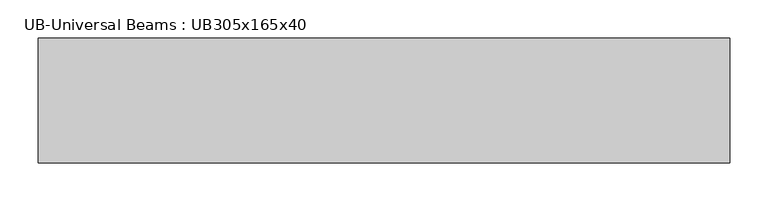
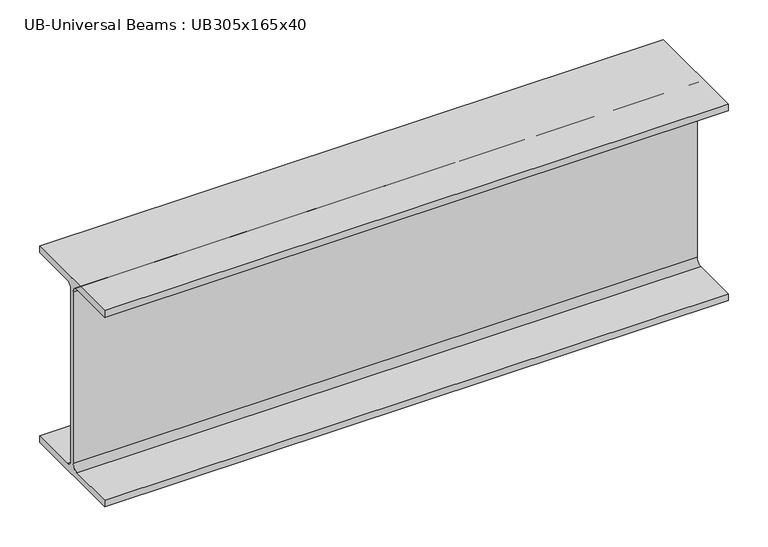
"""IFC4 building model written with IfcOpenShell, lengths in millimetres: beam geometry, UB-Universal Beams : UB305x165x40."""

from ifc_helpers import new_model, si_unit, point, frame, frame_2d, origin, place, context, project, spatial, polyline, circle_curve, trimmed, segment, composite_curve, outline, extrude, source, transform, mapped, element, save


def ub_universal_beams_ub305x165x40_7500c72c(model_context):
    return source(origin(), model_context, "Body", "SweptSolid", [
        extrude(outline(composite_curve([segment(polyline([(82.5, -141.5), (82.5, -151.7), (-82.5, -151.7), (-82.5, -141.5), (-11.9, -141.5)]), True, "CONTINUOUS"), segment(trimmed(circle_curve(frame_2d((-11.9, -132.6)), 8.9), [point((-11.9, -141.5))], [point((-3.0, -132.6))], True, "CARTESIAN"), True, "CONTINUOUS"), segment(polyline([(-3.0, -132.6), (-3.0, 132.6)]), True, "CONTINUOUS"), segment(trimmed(circle_curve(frame_2d((-11.9, 132.6)), 8.9), [point((-3.0, 132.6))], [point((-11.9, 141.5))], True, "CARTESIAN"), True, "CONTINUOUS"), segment(polyline([(-11.9, 141.5), (-82.5, 141.5), (-82.5, 151.7), (82.5, 151.7), (82.5, 141.5), (11.9, 141.5)]), True, "CONTINUOUS"), segment(trimmed(circle_curve(frame_2d((11.9, 132.6)), 8.9), [point((11.9, 141.5))], [point((3.0, 132.6))], True, "CARTESIAN"), True, "CONTINUOUS"), segment(polyline([(3.0, 132.6), (3.0, -132.6)]), True, "CONTINUOUS"), segment(trimmed(circle_curve(frame_2d((11.9, -132.6)), 8.9), [point((3.0, -132.6))], [point((11.9, -141.5))], True, "CARTESIAN"), True, "CONTINUOUS"), segment(polyline([(11.9, -141.5), (82.5, -141.5)]), True, "CONTINUOUS")], self_intersect=False)), frame((175.9, 0.0, 0.0), z_axis=(1.0, 0.0, 0.0), x_axis=(0.0, 1.0, 0.0)), (0.0, 0.0, 1.0), 910.4),
    ])


if __name__ == "__main__":
    model = new_model("IFC4")
    model_context = context("Model", 3, world=origin())
    ifc_project = project(units=[si_unit("LENGTHUNIT", "METRE", prefix="MILLI")], contexts=[model_context])
    site = spatial("IfcSite", under=ifc_project)
    building = spatial("IfcBuilding", under=site)
    placement = place(None, origin())
    ub_universal_beams_ub305x165x40_shape = ub_universal_beams_ub305x165x40_7500c72c(model_context)
    element("IfcBeam", 1, ObjectType="UB-Universal Beams : UB305x165x40", at=placement, inside=building, context=model_context, shape_type="MappedRepresentation", body=[
        mapped(ub_universal_beams_ub305x165x40_shape, transform((0.0, 0.0, 0.0), x_axis=(1.0, 0.0, 0.0), y_axis=(0.0, 1.0, 0.0), z_axis=(0.0, 0.0, 1.0))),
    ])
    save(model, "model.ifc")

# Revit data of these elements
# Type "UB-Universal Beams : UB305x165x40"
#   Section Name Key = "UB305X165X40"
#   Width = 16.5 cm
#   Web Thickness = 0.6 cm
#   Web Fillet = 0.89 cm
#   Warping Constant = 164000.0 cm⁶
#   Torsional Moment of Inertia = 14.70 cm⁴
#   Section Area = 51.3 cm²
#   Plastic Modulus weak axis = 142.0 cm³
#   Plastic Modulus strong axis = 623.0 cm³
#   Nominal Weight = 40.2999 kgf/m
#   Moment of Inertia weak axis = 764.00 cm⁴
#   Moment of Inertia strong axis = 8503.00 cm⁴
#   Height = 30.34 cm
#   Flange Thickness = 1.02 cm
#   Elastic Modulus weak axis = 92.6 cm³
#   Elastic Modulus strong axis = 560.0 cm³
#   Centroid Vertical = 15.17 cm
#   Centroid Horizontal = 8.25 cm
#   Bolt Spacing = 9.0 cm
#   Length [instance default] = 1500 mm
#   Structural Material [instance default] = Metal - Steel 43-275
#   Type Comments = ""
#   Assembly Code = ""
# Element 1 (IfcBeam, "UB-Universal Beams : UB305x165x40")
#   Materials on its faces: "Metal - Steel 43-275"
# Materials
#   "Metal - Steel 43-275": class "Metal", colour RGB 247 247 247, transparency 0, Cost = 0
